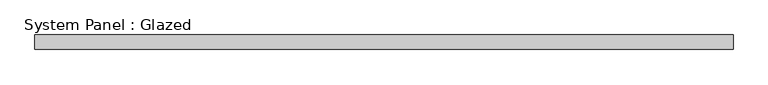
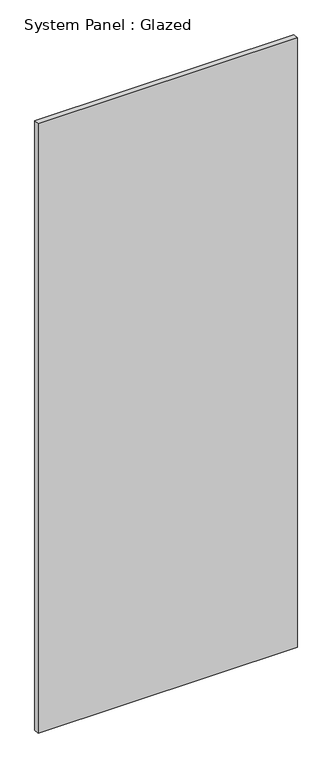
"""IFC4 building model written with IfcOpenShell, lengths in millimetres: plate geometry, System Panel : Glazed."""

from ifc_helpers import new_model, si_unit, origin, origin_with_axes, place, context, project, spatial, polyline, outline, extrude, source, transform, mapped, element, save


def system_panel_glazed_fbb400a4(model_context):
    return source(origin(), model_context, "Body", "SweptSolid", [
        extrude(outline(polyline([(604.4458489, 24.5), (-604.4458489, 24.5), (-604.4458489, 49.5), (604.4458489, 49.5), (604.4458489, 24.5)])), origin_with_axes(), (0.0, 0.0, 1.0), 3000.0),
    ])


if __name__ == "__main__":
    model = new_model("IFC4")
    model_context = context("Model", 3, world=origin())
    ifc_project = project(units=[si_unit("LENGTHUNIT", "METRE", prefix="MILLI")], contexts=[model_context])
    site = spatial("IfcSite", under=ifc_project)
    building = spatial("IfcBuilding", under=site)
    placement = place(None, origin())
    system_panel_glazed_shape = system_panel_glazed_fbb400a4(model_context)
    element("IfcPlate", 1, ObjectType="System Panel : Glazed", at=placement, inside=building, context=model_context, shape_type="MappedRepresentation", body=[
        mapped(system_panel_glazed_shape, transform((0.0, 0.0, 0.0), x_axis=(1.0, 0.0, 0.0), y_axis=(0.0, 1.0, 0.0), z_axis=(0.0, 0.0, 1.0))),
    ])
    save(model, "model.ifc")

# Revit data of these elements
# Type "System Panel : Glazed"
#   Keynote = "H11"
#   Construction Type Id = "GSP4R"
#   Analytic Construction = "1/8 in Pilkington single glazing"
#   Visual Light Transmittance = 0.9
#   Solar Heat Gain Coefficient = 0.86
#   Heat Transfer Coefficient (U) = 6.7069 W/(m²·K)
#   Define Thermal Properties by = 1
# Element 1 (IfcPlate, "System Panel : Glazed")
#   Materials on its faces: "Glass"
# Materials
#   "Glass": class "Glass", colour RGB 0 128 192, transparency 0.9, Description = "Soda Lime Glass", Cost = 0
